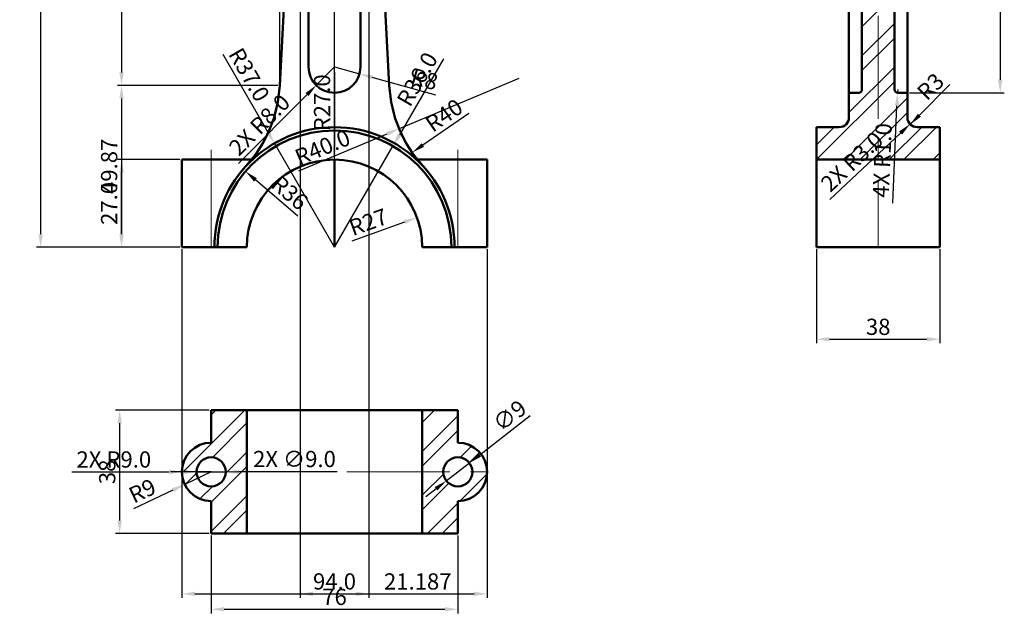
# Model space of a CAD drawing. Units: millimetres. Extents: x 3127 to 3430, y 1464 to 1830.
# Tile 1 of 2: x 3127 to 3430, y 1464 to 1647. Entities that reach past the tile are written whole.
import ezdxf

# ---------------------------------------------------------------- set-up
doc = ezdxf.new("R2010")
doc.units = ezdxf.units.MM
doc.linetypes.add('CENTER', pattern=[50.8, 31.75, -6.35, 6.35, -6.35])
for name, color, linetype, lineweight in [('M-CNTR', 1, 'CENTER', 18), ('M-DIMS', 2, 'Continuous', 25), ('M-HATC', 8, 'Continuous', 18), ('M-OUTL', 7, 'Continuous', 50)]:
    doc.layers.add(name, color=color, linetype=linetype, lineweight=lineweight)
doc.styles.get("Standard").update_dxf_attribs({"font": 'arial.ttf'})
doc.dimstyles.new('ISO-25', dxfattribs={"dimtxt": 5, "dimasz": 4, "dimexe": 1.25, "dimexo": 0.625, "dimtad": 1, "dimdsep": 46, "dimtxsty": 'Standard', "dimcen": 2.5, "dimadec": 0, "dimazin": 0, "dimtfac": 1, "dimtmove": 0, "dimatfit": 3, "dimfxl": 1, "dimarcsym": 0})

# ---------------------------------------------------------------- blocks, each defined once
blk = doc.blocks.new('*D1')
at = {"layer": 'Defpoints', "color": 0, "transparency": 16777216}
for p in [(3401.51, 1614.37), (3403.63, 1616.5)]:
    blk.add_point(p, dxfattribs=at)
at = {"layer": 'M-DIMS', "color": 0, "lineweight": -2, "transparency": 16777216}
blk.add_line((3413.75, 1626.62), (3404.34, 1617.2), dxfattribs=at)
at = {"layer": 'M-DIMS', "color": 0, "transparency": 16777216}
blk.add_solid([(3403.87, 1617.67), (3404.81, 1616.73), (3401.51, 1614.37)], dxfattribs=at)
at = {"layer": 'M-DIMS', "color": 0, "transparency": 16777216, "insert": (3408.21, 1625.57), "char_height": 5, "attachment_point": 5, "rotation": 45}
blk.add_mtext('R3', dxfattribs=at)
blk = doc.blocks.new('*D2')
at = {"layer": 'Defpoints', "color": 0, "transparency": 16777216}
for p in [(3372.63, 1576.5), (3410.63, 1576.5), (3410.63, 1548.12)]:
    blk.add_point(p, dxfattribs=at)
at = {"layer": 'M-DIMS', "color": 0, "lineweight": -2, "transparency": 16777216}
for p, q in [((3372.63, 1575.87), (3372.63, 1546.87)), ((3410.63, 1575.87), (3410.63, 1546.87)), ((3376.63, 1548.12), (3406.63, 1548.12))]:
    blk.add_line(p, q, dxfattribs=at)
at = {"layer": 'M-DIMS', "color": 0, "transparency": 16777216}
for points in [[(3376.63, 1548.78), (3376.63, 1547.45), (3372.63, 1548.12)], [(3406.63, 1548.78), (3406.63, 1547.45), (3410.63, 1548.12)]]:
    blk.add_solid(points, dxfattribs=at)
at = {"layer": 'M-DIMS', "color": 0, "transparency": 16777216, "insert": (3391.63, 1551.3), "char_height": 5, "attachment_point": 5}
blk.add_mtext('38', dxfattribs=at)
blk = doc.blocks.new('*D4')
at = {"layer": 'Defpoints', "color": 0, "transparency": 16777216}
for p in [(3186.15, 1488.22), (3262.15, 1488.22), (3262.15, 1464.86)]:
    blk.add_point(p, dxfattribs=at)
at = {"layer": 'M-DIMS', "color": 0, "lineweight": -2, "transparency": 16777216}
for p, q in [((3186.15, 1487.6), (3186.15, 1463.61)), ((3262.15, 1487.6), (3262.15, 1463.61)), ((3190.15, 1464.86), (3258.15, 1464.86))]:
    blk.add_line(p, q, dxfattribs=at)
at = {"layer": 'M-DIMS', "color": 0, "transparency": 16777216}
for points in [[(3190.15, 1465.53), (3190.15, 1464.2), (3186.15, 1464.86)], [(3258.15, 1465.53), (3258.15, 1464.2), (3262.15, 1464.86)]]:
    blk.add_solid(points, dxfattribs=at)
at = {"layer": 'M-DIMS', "color": 0, "transparency": 16777216, "insert": (3224.15, 1468.04), "char_height": 5, "attachment_point": 5}
blk.add_mtext('76', dxfattribs=at)
blk = doc.blocks.new('*D5')
at = {"layer": 'Defpoints', "color": 0, "transparency": 16777216}
for p in [(3186.15, 1526.22), (3157.96, 1488.22), (3186.15, 1488.22)]:
    blk.add_point(p, dxfattribs=at)
at = {"layer": 'M-DIMS', "color": 0, "lineweight": -2, "transparency": 16777216}
for p, q in [((3185.52, 1526.22), (3156.71, 1526.22)), ((3157.96, 1522.22), (3157.96, 1492.22)), ((3185.52, 1488.22), (3156.71, 1488.22))]:
    blk.add_line(p, q, dxfattribs=at)
at = {"layer": 'M-DIMS', "color": 0, "transparency": 16777216}
for points in [[(3157.29, 1522.22), (3158.63, 1522.22), (3157.96, 1526.22)], [(3157.29, 1492.22), (3158.63, 1492.22), (3157.96, 1488.22)]]:
    blk.add_solid(points, dxfattribs=at)
at = {"layer": 'M-DIMS', "color": 0, "transparency": 16777216, "insert": (3154.78, 1507.22), "char_height": 5, "attachment_point": 5, "rotation": 90}
blk.add_mtext('38', dxfattribs=at)
blk = doc.blocks.new('*D6')
at = {"layer": 'Defpoints', "color": 0, "transparency": 16777216}
for p in [(3186.15, 1507.22), (3178.02, 1503.36)]:
    blk.add_point(p, dxfattribs=at)
at = {"layer": 'M-DIMS', "color": 0, "lineweight": -2, "transparency": 16777216}
for p, q in [((3186.15, 1507.22), (3178.02, 1503.36)), ((3162.37, 1495.92), (3174.41, 1501.64))]:
    blk.add_line(p, q, dxfattribs=at)
at = {"layer": 'M-DIMS', "color": 0, "transparency": 16777216}
blk.add_solid([(3174.12, 1502.24), (3174.69, 1501.04), (3178.02, 1503.36)], dxfattribs=at)
at = {"layer": 'M-DIMS', "color": 0, "transparency": 16777216, "insert": (3165.22, 1500.79), "char_height": 5, "attachment_point": 5, "rotation": 25.423}
blk.add_mtext('R9', dxfattribs=at)
blk = doc.blocks.new('*D7')
at = {"layer": 'Defpoints', "color": 0, "transparency": 16777216}
for p in [(3265.71, 1509.98), (3258.59, 1504.47)]:
    blk.add_point(p, dxfattribs=at)
at = {"layer": 'M-DIMS', "color": 0, "lineweight": -2, "transparency": 16777216}
for p, q in [((3284.47, 1524.49), (3268.87, 1512.42)), ((3258.59, 1504.47), (3265.71, 1509.98)), ((3255.43, 1502.02), (3252.26, 1499.57))]:
    blk.add_line(p, q, dxfattribs=at)
at = {"layer": 'M-DIMS', "color": 0, "transparency": 16777216}
for points in [[(3268.46, 1512.95), (3269.28, 1511.9), (3265.71, 1509.98)], [(3255.02, 1502.55), (3255.83, 1501.49), (3258.59, 1504.47)]]:
    blk.add_solid(points, dxfattribs=at)
at = {"layer": 'M-DIMS', "color": 0, "transparency": 16777216, "insert": (3278.5, 1524.06), "char_height": 5, "attachment_point": 5, "rotation": 37.7248}
blk.add_mtext('∅9', dxfattribs=at)
blk = doc.blocks.new('*D8')
at = {"layer": 'Defpoints', "color": 0, "transparency": 16777216}
for p in [(3249.56, 1585.63), (3224.15, 1576.5)]:
    blk.add_point(p, dxfattribs=at)
at = {"layer": 'M-DIMS', "color": 0, "lineweight": -2, "transparency": 16777216}
blk.add_line((3229.61, 1578.46), (3245.79, 1584.28), dxfattribs=at)
at = {"layer": 'M-DIMS', "color": 0, "transparency": 16777216}
blk.add_solid([(3245.57, 1584.9), (3246.02, 1583.65), (3249.56, 1585.63)], dxfattribs=at)
at = {"layer": 'M-DIMS', "color": 0, "transparency": 16777216, "insert": (3234.76, 1583.64), "char_height": 5, "attachment_point": 5, "rotation": 19.7728}
blk.add_mtext('R27', dxfattribs=at)
blk = doc.blocks.new('*D9')
at = {"layer": 'Defpoints', "color": 0, "transparency": 16777216}
for p in [(3196.75, 1599.85), (3224.15, 1576.5)]:
    blk.add_point(p, dxfattribs=at)
at = {"layer": 'M-DIMS', "color": 0, "lineweight": -2, "transparency": 16777216}
blk.add_line((3212.88, 1586.1), (3199.79, 1597.25), dxfattribs=at)
at = {"layer": 'M-DIMS', "color": 0, "transparency": 16777216}
blk.add_solid([(3200.23, 1597.76), (3199.36, 1596.74), (3196.75, 1599.85)], dxfattribs=at)
at = {"layer": 'M-DIMS', "color": 0, "transparency": 16777216, "insert": (3209.92, 1592.8), "char_height": 5, "attachment_point": 5, "rotation": 319.5625}
blk.add_mtext('R36', dxfattribs=at)
blk = doc.blocks.new('*D10')
at = {"layer": 'Defpoints', "color": 0, "transparency": 16777216}
for p in [(3224.15, 1632.1), (3231.85, 1629.94)]:
    blk.add_point(p, dxfattribs=at)
at = {"layer": 'M-DIMS', "color": 0, "lineweight": -2, "transparency": 16777216}
for p, q in [((3224.15, 1632.1), (3231.85, 1629.94)), ((3255.34, 1623.37), (3235.71, 1628.86))]:
    blk.add_line(p, q, dxfattribs=at)
at = {"layer": 'M-DIMS', "color": 0, "transparency": 16777216}
blk.add_solid([(3235.88, 1629.51), (3235.53, 1628.22), (3231.85, 1629.94)], dxfattribs=at)
at = {"layer": 'M-DIMS', "color": 0, "transparency": 16777216, "insert": (3251.71, 1627.69), "char_height": 5, "attachment_point": 5, "rotation": 344.3775}
blk.add_mtext('R8', dxfattribs=at)
blk = doc.blocks.new('*D11')
at = {"layer": 'Defpoints', "color": 0, "transparency": 16777216}
for p in [(3280.97, 1628.46), (3248.08, 1605.7)]:
    blk.add_point(p, dxfattribs=at)
at = {"layer": 'M-DIMS', "color": 0, "lineweight": -2, "transparency": 16777216}
blk.add_line((3265.49, 1617.75), (3251.36, 1607.98), dxfattribs=at)
at = {"layer": 'M-DIMS', "color": 0, "transparency": 16777216}
blk.add_solid([(3250.99, 1608.53), (3251.74, 1607.43), (3248.08, 1605.7)], dxfattribs=at)
at = {"layer": 'M-DIMS', "color": 0, "transparency": 16777216, "insert": (3258.26, 1616.62), "char_height": 5, "attachment_point": 5, "rotation": 34.6821}
blk.add_mtext('R40', dxfattribs=at)
blk = doc.blocks.new('*D12')
at = {"layer": 'Defpoints', "color": 0, "transparency": 16777216}
for p in [(3213.56, 1746.21), (3234.74, 1746.21), (3219.51, 1682.41), (3207.27, 1626.37), (3241.02, 1626.37)]:
    blk.add_point(p, dxfattribs=at)
at = {"layer": 'M-DIMS', "color": 0, "lineweight": -2, "transparency": 16777216}
blk.add_arc((3224.15, 1948.35), 265.98, 267.8617, 272.1383, dxfattribs=at)
at = {"layer": 'M-DIMS', "color": 0, "transparency": 16777216}
for points in [[(3214.19, 1681.89), (3214.25, 1683.22), (3210.23, 1682.73)], [(3234.04, 1683.22), (3234.1, 1681.89), (3238.07, 1682.73)]]:
    blk.add_solid(points, dxfattribs=at)
at = {"layer": 'M-DIMS', "color": 0, "transparency": 16777216, "insert": (3224.15, 1685.55), "char_height": 5, "attachment_point": 5}
blk.add_mtext('6°', dxfattribs=at)
blk = doc.blocks.new('*D16')
at = {"layer": 'Defpoints', "color": 0, "transparency": 16777216}
for p in [(3224.15, 1777.7), (3133.63, 1576.5), (3177.15, 1576.5)]:
    blk.add_point(p, dxfattribs=at)
at = {"layer": 'M-DIMS', "color": 0, "lineweight": -2, "transparency": 16777216}
for p, q in [((3223.52, 1777.7), (3132.38, 1777.7)), ((3133.63, 1773.7), (3133.63, 1580.5)), ((3176.52, 1576.5), (3132.38, 1576.5))]:
    blk.add_line(p, q, dxfattribs=at)
at = {"layer": 'M-DIMS', "color": 0, "transparency": 16777216}
for points in [[(3132.96, 1773.7), (3134.3, 1773.7), (3133.63, 1777.7)], [(3132.96, 1580.5), (3134.3, 1580.5), (3133.63, 1576.5)]]:
    blk.add_solid(points, dxfattribs=at)
at = {"layer": 'M-DIMS', "color": 0, "transparency": 16777216, "insert": (3130.45, 1677.1), "char_height": 5, "attachment_point": 5, "rotation": 90}
blk.add_mtext('201.2', dxfattribs=at)
blk = doc.blocks.new('*D20')
at = {"layer": 'Defpoints', "color": 0, "transparency": 16777216}
for p in [(3177.15, 1576.5), (3271.15, 1576.5), (3271.15, 1469.62)]:
    blk.add_point(p, dxfattribs=at)
at = {"layer": 'M-DIMS', "color": 0, "lineweight": -2, "transparency": 16777216}
for p, q in [((3177.15, 1575.87), (3177.15, 1468.37)), ((3271.15, 1575.87), (3271.15, 1468.37)), ((3181.15, 1469.62), (3267.15, 1469.62))]:
    blk.add_line(p, q, dxfattribs=at)
at = {"layer": 'M-DIMS', "color": 0, "transparency": 16777216}
for points in [[(3181.15, 1470.29), (3181.15, 1468.96), (3177.15, 1469.62)], [(3267.15, 1470.29), (3267.15, 1468.96), (3271.15, 1469.62)]]:
    blk.add_solid(points, dxfattribs=at)
at = {"layer": 'M-DIMS', "color": 0, "transparency": 16777216, "insert": (3224.15, 1472.8), "char_height": 5, "attachment_point": 5}
blk.add_mtext('94.0', dxfattribs=at)
blk = doc.blocks.new('*D21')
at = {"layer": 'Defpoints', "color": 0, "transparency": 16777216}
for p in [(3158.55, 1603.5), (3177.15, 1603.5), (3177.15, 1576.5)]:
    blk.add_point(p, dxfattribs=at)
at = {"layer": 'M-DIMS', "color": 0, "lineweight": -2, "transparency": 16777216}
for p, q in [((3176.52, 1603.5), (3157.3, 1603.5)), ((3158.55, 1580.5), (3158.55, 1599.5)), ((3176.52, 1576.5), (3157.3, 1576.5))]:
    blk.add_line(p, q, dxfattribs=at)
at = {"layer": 'M-DIMS', "color": 0, "transparency": 16777216}
for points in [[(3157.88, 1599.5), (3159.22, 1599.5), (3158.55, 1603.5)], [(3157.88, 1580.5), (3159.22, 1580.5), (3158.55, 1576.5)]]:
    blk.add_solid(points, dxfattribs=at)
at = {"layer": 'M-DIMS', "color": 0, "transparency": 16777216, "insert": (3155.37, 1590), "char_height": 5, "attachment_point": 5, "rotation": 90}
blk.add_mtext('27.0', dxfattribs=at)
blk = doc.blocks.new('*D23')
at = {"layer": 'Defpoints', "color": 0, "transparency": 16777216}
for p in [(3400.63, 1730.1), (3400.63, 1624.1), (3429.23, 1624.1)]:
    blk.add_point(p, dxfattribs=at)
at = {"layer": 'M-DIMS', "color": 0, "lineweight": -2, "transparency": 16777216}
for p, q in [((3401.25, 1730.1), (3430.48, 1730.1)), ((3429.23, 1726.1), (3429.23, 1628.1)), ((3401.25, 1624.1), (3430.48, 1624.1))]:
    blk.add_line(p, q, dxfattribs=at)
at = {"layer": 'M-DIMS', "color": 0, "transparency": 16777216}
for points in [[(3428.56, 1726.1), (3429.9, 1726.1), (3429.23, 1730.1)], [(3428.56, 1628.1), (3429.9, 1628.1), (3429.23, 1624.1)]]:
    blk.add_solid(points, dxfattribs=at)
at = {"layer": 'M-DIMS', "color": 0, "transparency": 16777216, "insert": (3426.05, 1677.1), "char_height": 5, "attachment_point": 5, "rotation": 90}
blk.add_mtext('106.0', dxfattribs=at)
blk = doc.blocks.new('*D24')
at = {"layer": 'Defpoints', "color": 0, "transparency": 16777216}
for p in [(3213.56, 1746.21), (3234.74, 1746.21), (3234.74, 1469.62)]:
    blk.add_point(p, dxfattribs=at)
at = {"layer": 'M-DIMS', "color": 0, "lineweight": -2, "transparency": 16777216}
for p, q in [((3213.56, 1745.59), (3213.56, 1468.37)), ((3234.74, 1745.59), (3234.74, 1468.37)), ((3217.56, 1469.62), (3230.74, 1469.62)), ((3234.74, 1469.62), (3260.83, 1469.62))]:
    blk.add_line(p, q, dxfattribs=at)
at = {"layer": 'M-DIMS', "color": 0, "transparency": 16777216}
for points in [[(3217.56, 1470.29), (3217.56, 1468.96), (3213.56, 1469.62)], [(3230.74, 1470.29), (3230.74, 1468.96), (3234.74, 1469.62)]]:
    blk.add_solid(points, dxfattribs=at)
at = {"layer": 'M-DIMS', "color": 0, "transparency": 16777216, "insert": (3249.79, 1472.8), "char_height": 5, "attachment_point": 5}
blk.add_mtext('21.187', dxfattribs=at)
blk = doc.blocks.new('*D25')
at = {"layer": 'Defpoints', "color": 0, "transparency": 16777216}
for p in [(3224.15, 1818.8), (3207.27, 1626.37), (3224.15, 1603.5)]:
    blk.add_point(p, dxfattribs=at)
at = {"layer": 'M-DIMS', "color": 0, "lineweight": -2, "transparency": 16777216}
for p, q in [((3207.27, 1626.99), (3207.27, 1820.05)), ((3224.15, 1604.12), (3224.15, 1820.05)), ((3211.27, 1818.8), (3220.15, 1818.8)), ((3224.15, 1818.8), (3249.66, 1818.8))]:
    blk.add_line(p, q, dxfattribs=at)
at = {"layer": 'M-DIMS', "color": 0, "transparency": 16777216}
for points in [[(3211.27, 1819.46), (3211.27, 1818.13), (3207.27, 1818.8)], [(3220.15, 1819.46), (3220.15, 1818.13), (3224.15, 1818.8)]]:
    blk.add_solid(points, dxfattribs=at)
at = {"layer": 'M-DIMS', "color": 0, "transparency": 16777216, "insert": (3238.91, 1821.97), "char_height": 5, "attachment_point": 5}
blk.add_mtext('16.874', dxfattribs=at)
blk = doc.blocks.new('*D26')
at = {"layer": 'Defpoints', "color": 0, "transparency": 16777216}
for p in [(3213.56, 1746.21), (3158.55, 1626.37), (3207.27, 1626.37)]:
    blk.add_point(p, dxfattribs=at)
at = {"layer": 'M-DIMS', "color": 0, "lineweight": -2, "transparency": 16777216}
for p, q in [((3212.93, 1746.21), (3157.3, 1746.21)), ((3158.55, 1742.21), (3158.55, 1630.37)), ((3206.65, 1626.37), (3157.3, 1626.37))]:
    blk.add_line(p, q, dxfattribs=at)
at = {"layer": 'M-DIMS', "color": 0, "transparency": 16777216}
for points in [[(3157.88, 1742.21), (3159.22, 1742.21), (3158.55, 1746.21)], [(3157.88, 1630.37), (3159.22, 1630.37), (3158.55, 1626.37)]]:
    blk.add_solid(points, dxfattribs=at)
at = {"layer": 'M-DIMS', "color": 0, "transparency": 16777216, "insert": (3155.37, 1686.29), "char_height": 5, "attachment_point": 5, "rotation": 90}
blk.add_mtext('119.85', dxfattribs=at)
blk = doc.blocks.new('*D27')
at = {"layer": 'Defpoints', "color": 0, "transparency": 16777216}
for p in [(3207.27, 1626.37), (3158.55, 1576.5), (3177.15, 1576.5)]:
    blk.add_point(p, dxfattribs=at)
at = {"layer": 'M-DIMS', "color": 0, "lineweight": -2, "transparency": 16777216}
for p, q in [((3206.65, 1626.37), (3157.3, 1626.37)), ((3158.55, 1622.37), (3158.55, 1580.5)), ((3176.52, 1576.5), (3157.3, 1576.5))]:
    blk.add_line(p, q, dxfattribs=at)
at = {"layer": 'M-DIMS', "color": 0, "transparency": 16777216}
for points in [[(3157.88, 1622.37), (3159.22, 1622.37), (3158.55, 1626.37)], [(3157.88, 1580.5), (3159.22, 1580.5), (3158.55, 1576.5)]]:
    blk.add_solid(points, dxfattribs=at)
at = {"layer": 'M-DIMS', "color": 0, "transparency": 16777216, "insert": (3155.37, 1601.43), "char_height": 5, "attachment_point": 5, "rotation": 90}
blk.add_mtext('49.87', dxfattribs=at)
blk = doc.blocks.new('*D31')
at = {"layer": 'Defpoints', "color": 0, "transparency": 16777216}
for p in [(3224.15, 1632.1), (3218.52, 1626.42)]:
    blk.add_point(p, dxfattribs=at)
at = {"layer": 'M-DIMS', "color": 0, "lineweight": -2, "transparency": 16777216}
for p, q in [((3224.15, 1632.1), (3218.52, 1626.42)), ((3194.61, 1602.31), (3215.7, 1623.58))]:
    blk.add_line(p, q, dxfattribs=at)
at = {"layer": 'M-DIMS', "color": 0, "transparency": 16777216}
blk.add_solid([(3215.23, 1624.04), (3216.17, 1623.11), (3218.52, 1626.42)], dxfattribs=at)
at = {"layer": 'M-DIMS', "color": 0, "transparency": 16777216, "insert": (3201.49, 1613.76), "char_height": 5, "attachment_point": 5, "rotation": 45.2377}
blk.add_mtext('2X R8.0', dxfattribs=at)
blk = doc.blocks.new('*D32')
at = {"layer": 'Defpoints', "color": 0, "transparency": 16777216}
for p in [(3280.97, 1628.46), (3244.07, 1613.01)]:
    blk.add_point(p, dxfattribs=at)
at = {"layer": 'M-DIMS', "color": 0, "lineweight": -2, "transparency": 16777216}
for p, q in [((3280.97, 1628.46), (3244.07, 1613.01)), ((3213.17, 1600.07), (3240.38, 1611.47))]:
    blk.add_line(p, q, dxfattribs=at)
at = {"layer": 'M-DIMS', "color": 0, "transparency": 16777216}
blk.add_solid([(3240.13, 1612.08), (3240.64, 1610.85), (3244.07, 1613.01)], dxfattribs=at)
at = {"layer": 'M-DIMS', "color": 0, "transparency": 16777216, "insert": (3220.71, 1606.67), "char_height": 5, "attachment_point": 5, "rotation": 22.7235}
blk.add_mtext('R40.0', dxfattribs=at)
blk = doc.blocks.new('*D33')
at = {"layer": 'Defpoints', "color": 0, "transparency": 16777216}
for p in [(3205.65, 1608.54), (3224.15, 1576.5)]:
    blk.add_point(p, dxfattribs=at)
at = {"layer": 'M-DIMS', "color": 0, "lineweight": -2, "transparency": 16777216}
for p, q in [((3189.8, 1636), (3203.65, 1612)), ((3224.15, 1576.5), (3205.65, 1608.54))]:
    blk.add_line(p, q, dxfattribs=at)
at = {"layer": 'M-DIMS', "color": 0, "transparency": 16777216}
blk.add_solid([(3204.23, 1612.34), (3203.07, 1611.67), (3205.65, 1608.54)], dxfattribs=at)
at = {"layer": 'M-DIMS', "color": 0, "transparency": 16777216, "insert": (3197.3, 1629.36), "char_height": 5, "attachment_point": 5, "rotation": 299.9971}
blk.add_mtext('R37.0', dxfattribs=at)
blk = doc.blocks.new('*D34')
at = {"layer": 'Defpoints', "color": 0, "transparency": 16777216}
for p in [(3242.15, 1607.67), (3224.15, 1576.5)]:
    blk.add_point(p, dxfattribs=at)
at = {"layer": 'M-DIMS', "color": 0, "lineweight": -2, "transparency": 16777216}
for p, q in [((3257.7, 1634.61), (3244.15, 1611.14)), ((3224.15, 1576.5), (3242.15, 1607.67))]:
    blk.add_line(p, q, dxfattribs=at)
at = {"layer": 'M-DIMS', "color": 0, "transparency": 16777216}
blk.add_solid([(3243.57, 1611.47), (3244.72, 1610.8), (3242.15, 1607.67)], dxfattribs=at)
at = {"layer": 'M-DIMS', "color": 0, "transparency": 16777216, "insert": (3250.19, 1627.97), "char_height": 5, "attachment_point": 5, "rotation": 60.004}
blk.add_mtext('R36.0', dxfattribs=at)
blk = doc.blocks.new('*D35')
at = {"layer": 'Defpoints', "color": 0, "transparency": 16777216}
for p in [(3224.15, 1603.5), (3224.15, 1576.5)]:
    blk.add_point(p, dxfattribs=at)
at = {"layer": 'M-DIMS', "color": 0, "lineweight": -2, "transparency": 16777216}
for p, q in [((3224.15, 1630.5), (3224.15, 1607.5)), ((3224.15, 1576.5), (3224.15, 1603.5))]:
    blk.add_line(p, q, dxfattribs=at)
at = {"layer": 'M-DIMS', "color": 0, "transparency": 16777216}
blk.add_solid([(3223.48, 1607.5), (3224.82, 1607.5), (3224.15, 1603.5)], dxfattribs=at)
at = {"layer": 'M-DIMS', "color": 0, "transparency": 16777216, "insert": (3220.97, 1621), "char_height": 5, "attachment_point": 5, "rotation": 89.9992}
blk.add_mtext('R27.0', dxfattribs=at)
blk = doc.blocks.new('*D36')
at = {"layer": 'Defpoints', "color": 0, "transparency": 16777216}
for p in [(3177.15, 1507.22), (3186.15, 1507.22)]:
    blk.add_point(p, dxfattribs=at)
at = {"layer": 'M-DIMS', "color": 0, "lineweight": -2, "transparency": 16777216}
for p, q in [((3143.2, 1507.22), (3173.15, 1507.22)), ((3186.15, 1507.22), (3177.15, 1507.22))]:
    blk.add_line(p, q, dxfattribs=at)
at = {"layer": 'M-DIMS', "color": 0, "transparency": 16777216}
blk.add_solid([(3173.15, 1507.89), (3173.15, 1506.56), (3177.15, 1507.22)], dxfattribs=at)
at = {"layer": 'M-DIMS', "color": 0, "transparency": 16777216, "insert": (3156.17, 1510.4), "char_height": 5, "attachment_point": 5, "rotation": 359.9991}
blk.add_mtext('2X R9.0', dxfattribs=at)
blk = doc.blocks.new('*D37')
at = {"layer": 'Defpoints', "color": 0, "transparency": 16777216}
for p in [(3181.65, 1507.22), (3190.65, 1507.22)]:
    blk.add_point(p, dxfattribs=at)
at = {"layer": 'M-DIMS', "color": 0, "lineweight": -2, "transparency": 16777216}
for p, q in [((3177.65, 1507.22), (3173.65, 1507.22)), ((3181.65, 1507.22), (3190.65, 1507.22)), ((3224.99, 1507.22), (3194.65, 1507.22))]:
    blk.add_line(p, q, dxfattribs=at)
at = {"layer": 'M-DIMS', "color": 0, "transparency": 16777216}
for points in [[(3177.65, 1507.89), (3177.65, 1506.55), (3181.65, 1507.22)], [(3194.65, 1507.89), (3194.65, 1506.56), (3190.65, 1507.22)]]:
    blk.add_solid(points, dxfattribs=at)
at = {"layer": 'M-DIMS', "color": 0, "transparency": 16777216, "insert": (3211.82, 1510.54), "char_height": 5, "attachment_point": 5, "rotation": 0.0018}
blk.add_mtext('2X ∅9.0', dxfattribs=at)
blk = doc.blocks.new('*D38')
at = {"layer": 'Defpoints', "color": 0, "transparency": 16777216}
for p in [(3401.44, 1614.44), (3403.63, 1616.5)]:
    blk.add_point(p, dxfattribs=at)
at = {"layer": 'M-DIMS', "color": 0, "lineweight": -2, "transparency": 16777216}
for p, q in [((3403.63, 1616.5), (3401.44, 1614.44)), ((3376.71, 1591.19), (3398.53, 1611.7))]:
    blk.add_line(p, q, dxfattribs=at)
at = {"layer": 'M-DIMS', "color": 0, "transparency": 16777216}
blk.add_solid([(3398.07, 1612.19), (3398.99, 1611.22), (3401.44, 1614.44)], dxfattribs=at)
at = {"layer": 'M-DIMS', "color": 0, "transparency": 16777216, "insert": (3383.98, 1602.39), "char_height": 5, "attachment_point": 5, "rotation": 43.2283}
blk.add_mtext('2X R3.0', dxfattribs=at)
blk = doc.blocks.new('*D39')
at = {"layer": 'Defpoints', "color": 0, "transparency": 16777216}
for p in [(3397.59, 1624.1), (3397.63, 1625.1)]:
    blk.add_point(p, dxfattribs=at)
at = {"layer": 'M-DIMS', "color": 0, "lineweight": -2, "transparency": 16777216}
for p, q in [((3397.63, 1625.1), (3397.59, 1624.1)), ((3396.14, 1590.06), (3397.42, 1620.1))]:
    blk.add_line(p, q, dxfattribs=at)
at = {"layer": 'M-DIMS', "color": 0, "transparency": 16777216}
blk.add_solid([(3396.75, 1620.13), (3398.08, 1620.07), (3397.59, 1624.1)], dxfattribs=at)
at = {"layer": 'M-DIMS', "color": 0, "transparency": 16777216, "insert": (3393.52, 1603.22), "char_height": 5, "attachment_point": 5, "rotation": 87.5733}
blk.add_mtext('4X R1.0', dxfattribs=at)

msp = doc.modelspace()

# ---------------------------------------------------------------- hatches: boundary and pattern name
at = {"layer": 'M-HATC'}
h = msp.add_hatch(dxfattribs=at)
h.set_pattern_fill('ANSI32', color=256)
h.paths.add_polyline_path([(3391.6295, 1800.1957), (3372.6295, 1800.1957), (3372.6295, 1794.5957), (3391.6295, 1794.5957)])
h.paths.add_polyline_path([(3410.6295, 1800.1957), (3391.6295, 1800.1957), (3391.6295, 1794.5957), (3410.6295, 1794.5957)])
h.paths.add_polyline_path([(3400.6295, 1755.1957), (3410.6295, 1755.1957), (3410.6295, 1760.7957), (3391.6295, 1760.7957), (3391.6295, 1603.4957), (3410.6295, 1603.4957), (3410.6295, 1613.4957), (3403.6295, 1613.4957, -0.41421356), (3400.6295, 1616.4957), (3400.6295, 1624.0957), (3397.6295, 1624.0957, -0.41421356), (3396.6295, 1625.0957), (3396.6295, 1729.0957, -0.41421356), (3397.6295, 1730.0957), (3400.6295, 1730.0957)])
h.paths.add_polyline_path([(3391.6295, 1760.7957), (3372.6295, 1760.7957), (3372.6295, 1755.1957), (3382.6295, 1755.1957), (3382.6295, 1730.0957), (3385.6295, 1730.0957, -0.41421356), (3386.6295, 1729.0957), (3386.6295, 1625.0957, -0.41421356), (3385.6295, 1624.0957), (3382.6295, 1624.0957), (3382.6295, 1616.4957, -0.41421356), (3379.6295, 1613.4957), (3372.6295, 1613.4957), (3372.6295, 1603.4957), (3391.6295, 1603.4957)])
h.paths.add_polyline_path([(3262.1486, 1526.2219), (3251.1486, 1526.2219), (3251.1486, 1507.2219), (3257.6486, 1507.2219, -1), (3266.6486, 1507.2219), (3271.1486, 1507.2219, 0.41421356), (3262.1486, 1516.2219)])
h.paths.add_polyline_path([(3271.1486, 1507.2219), (3266.6486, 1507.2219, -1), (3257.6486, 1507.2219), (3251.1486, 1507.2219), (3251.1486, 1488.2219), (3262.1486, 1488.2219), (3262.1486, 1498.2219, 0.41421356)])
h.paths.add_polyline_path([(3197.1486, 1526.2219), (3186.1486, 1526.2219), (3186.1486, 1516.2219, 0.41421356), (3177.1486, 1507.2219), (3181.6486, 1507.2219, -1), (3190.6486, 1507.2219), (3197.1486, 1507.2219)])
h.paths.add_polyline_path([(3197.1486, 1507.2219), (3190.6486, 1507.2219, -1), (3181.6486, 1507.2219), (3177.1486, 1507.2219, 0.41421356), (3186.1486, 1498.2219), (3186.1486, 1488.2219), (3197.1486, 1488.2219)])

# ---------------------------------------------------------------- linework, layer by layer
at = {"layer": 'M-CNTR'}
for p, q in [((3391.6295, 1800.1957), (3391.6295, 1576.4957)), ((3224.1486, 1777.6957), (3224.1486, 1624.0957)), ((3224.1486, 1624.0957), (3224.1486, 1576.4957)), ((3186.1486, 1576.4957), (3186.1486, 1606.4957)), ((3262.1486, 1576.4957), (3262.1486, 1606.4957)), ((3177.1486, 1507.2219), (3271.1486, 1507.2219))]:
    msp.add_line(p, q, dxfattribs=at)
at = {"layer": 'M-OUTL'}
for p, q in [((3382.6295, 1755.1957), (3382.6295, 1616.4957)), ((3400.6295, 1755.1957), (3400.6295, 1616.4957)), ((3213.5551, 1746.2148), (3207.2742, 1626.369)), ((3234.7422, 1746.2148), (3241.023, 1626.369)), ((3386.6295, 1729.0957), (3386.6295, 1625.0957)), ((3396.6295, 1729.0957), (3396.6295, 1625.0957)), ((3216.1486, 1722.0957), (3216.1486, 1632.0957)), ((3232.1486, 1722.0957), (3232.1486, 1632.0957)), ((3382.6295, 1624.0957), (3385.6295, 1624.0957)), ((3397.6295, 1624.0957), (3400.6295, 1624.0957)), ((3372.6295, 1613.4957), (3372.6295, 1576.4957)), ((3372.6295, 1613.4957), (3379.6295, 1613.4957)), ((3403.6295, 1613.4957), (3410.6295, 1613.4957)), ((3410.6295, 1613.4957), (3410.6295, 1576.4957)), ((3177.1486, 1576.4957), (3177.1486, 1603.4957)), ((3177.1486, 1603.4957), (3198.5807, 1603.4957)), ((3224.1486, 1576.4957), (3224.1486, 1603.4957)), ((3249.7166, 1603.4957), (3271.1486, 1603.4957)), ((3249.7166, 1603.4957), (3271.1486, 1603.4957)), ((3271.1486, 1576.4957), (3271.1486, 1603.4957)), ((3372.6295, 1603.4957), (3410.6295, 1603.4957)), ((3177.1486, 1576.4957), (3197.1486, 1576.4957)), ((3187.1486, 1576.4957), (3197.1486, 1576.4957)), ((3251.1486, 1576.4957), (3261.1486, 1576.4957)), ((3251.1486, 1576.4957), (3271.1486, 1576.4957)), ((3251.1486, 1576.4957), (3271.1486, 1576.4957)), ((3372.6295, 1576.4957), (3410.6295, 1576.4957)), ((3186.1486, 1526.2219), (3262.1486, 1526.2219)), ((3186.1486, 1516.2219), (3186.1486, 1526.2219)), ((3197.1486, 1526.2219), (3197.1486, 1488.2219)), ((3251.1486, 1526.2219), (3251.1486, 1488.2219)), ((3262.1486, 1516.2219), (3262.1486, 1526.2219)), ((3186.1486, 1488.2219), (3186.1486, 1498.2219)), ((3262.1486, 1488.2219), (3262.1486, 1498.2219)), ((3186.1486, 1488.2219), (3262.1486, 1488.2219))]:
    msp.add_line(p, q, dxfattribs=at)
for centre in [(3186.1486, 1507.2219), (3262.1486, 1507.2219)]:
    msp.add_circle(centre, 4.5, dxfattribs=at)
for centre, radius, start, end in [((3224.1486, 1632.0957), 8, 180, 0), ((3167.3291, 1628.4624), 40, 317.554231, 357), ((3280.9682, 1628.4624), 40, 183, 222.445769), ((3385.6295, 1625.0957), 1, 270, 0), ((3397.6295, 1625.0957), 1, 180, 270), ((3379.6295, 1616.4957), 3, 270, 0), ((3403.6295, 1616.4957), 3, 180, 270), ((3224.1486, 1576.4957), 37, 0, 180), ((3224.1486, 1576.4957), 36, 0, 180), ((3224.1486, 1576.4957), 27, 0, 180), ((3186.1486, 1507.2219), 9, 90, 270), ((3262.1486, 1507.2219), 9, 270, 90)]:
    msp.add_arc(centre, radius, start, end, dxfattribs=at)

# ---------------------------------------------------------------- dimensions: what is measured, and where the dimension line sits
at = {"layer": 'M-DIMS'}
for base, p1, p2, override, picture, middle in [((3224.1486, 1818.7957), (3207.2742, 1626.369), (3224.1486, 1603.4957), {"dimdec": 3, "dimlfac": 1, "dimrnd": 0, "dimzin": 0, "dimdsep": 46, "dimlunit": 2}, '*D25', (3238.9067, 1821.9736)), ((3234.7422, 1469.6219), (3213.5551, 1746.2148), (3234.7422, 1746.2148), {"dimdec": 3, "dimlfac": 1, "dimrnd": 0, "dimzin": 0, "dimdsep": 46, "dimlunit": 2}, '*D24', (3249.7884, 1472.7997)), ((3271.1486, 1469.6219), (3177.1486, 1576.4957), (3271.1486, 1576.4957), {"dimdec": 1, "dimlfac": 1, "dimrnd": 0, "dimzin": 0, "dimdsep": 46, "dimlunit": 2}, '*D20', (3224.1486, 1472.7997)), ((3410.6295, 1548.117), (3372.6295, 1576.4957), (3410.6295, 1576.4957), {"dimclrd": 0, "dimclre": 0, "dimclrt": 0}, '*D2', (3391.6295, 1551.2966)), ((3262.1486, 1464.8644), (3186.1486, 1488.2219), (3262.1486, 1488.2219), {"dimclrd": 0, "dimclre": 0, "dimclrt": 0}, '*D4', (3224.1486, 1468.0423))]:
    dim = msp.add_linear_dim(base=base, p1=p1, p2=p2, dimstyle='ISO-25', override=override, dxfattribs=at)
    dim.commit()
    dim.dimension.update_dxf_attribs({"geometry": picture, "text_midpoint": middle})
for base, p1, p2, override, picture, middle in [((3133.6315, 1576.4957), (3224.1486, 1777.6957), (3177.1486, 1576.4957), {"dimclrd": 0, "dimclre": 0, "dimclrt": 0}, '*D16', (3130.4537, 1677.0957)), ((3158.5486, 1626.369), (3213.5551, 1746.2148), (3207.2742, 1626.369), {"dimdec": 2, "dimlfac": 1, "dimrnd": 0, "dimzin": 0, "dimdsep": 46, "dimlunit": 2}, '*D26', (3155.3708, 1686.2919)), ((3429.2295, 1624.0957), (3400.6295, 1730.0957), (3400.6295, 1624.0957), {"dimdec": 1, "dimlfac": 1, "dimrnd": 0, "dimzin": 0, "dimdsep": 46, "dimlunit": 2}, '*D23', (3426.0516, 1677.0957)), ((3158.5486, 1576.4957), (3207.2742, 1626.369), (3177.1486, 1576.4957), {"dimdec": 2, "dimlfac": 1, "dimrnd": 0, "dimzin": 0, "dimdsep": 46, "dimlunit": 2}, '*D27', (3155.3708, 1601.4323)), ((3158.5486, 1603.4957), (3177.1486, 1576.4957), (3177.1486, 1603.4957), {"dimdec": 1, "dimlfac": 1, "dimrnd": 0, "dimzin": 0, "dimdsep": 46, "dimlunit": 2}, '*D21', (3155.3708, 1589.9957)), ((3157.9612, 1488.2219), (3186.1486, 1526.2219), (3186.1486, 1488.2219), {"dimclrd": 0, "dimclre": 0, "dimclrt": 0}, '*D5', (3154.7816, 1507.2219))]:
    dim = msp.add_linear_dim(base=base, p1=p1, p2=p2, angle=90, dimstyle='ISO-25', override=override, dxfattribs=at)
    dim.commit()
    dim.dimension.update_dxf_attribs({"geometry": picture, "text_midpoint": middle})
dim = msp.add_angular_dim_2l(base=(3219.5066, 1682.4079), line1=((3234.7422, 1746.2148), (3241.023, 1626.369)), line2=((3213.5551, 1746.2148), (3207.2742, 1626.369)), dimstyle='ISO-25', override={"dimclrd": 0, "dimclre": 0, "dimclrt": 0}, dxfattribs=at)
dim.commit()
dim.dimension.update_dxf_attribs({"geometry": '*D12', "text_midpoint": (3224.1486, 1685.5453)})
for center, mpoint, override, picture, middle in [((3224.1486, 1576.4957), (3205.6502, 1608.5396), {"dimdec": 1, "dimlfac": 1, "dimrnd": 0, "dimzin": 0, "dimdsep": 46, "dimlunit": 2}, '*D33', (3194.5512, 1627.7659)), ((3224.1486, 1576.4957), (3242.1465, 1607.6739), {"dimdec": 1, "dimlfac": 1, "dimrnd": 0, "dimzin": 0, "dimdsep": 46, "dimlunit": 2}, '*D34', (3252.9452, 1626.3808)), ((3224.1486, 1632.0957), (3231.8531, 1629.9413), {"dimclrd": 0, "dimclre": 0, "dimclrt": 0}, '*D10', (3250.8507, 1624.629)), ((3403.6295, 1616.4957), (3401.5082, 1614.3744), {"dimclrd": 0, "dimclre": 0, "dimclrt": 0}, '*D1', (3410.4576, 1623.3238)), ((3280.9682, 1628.4624), (3244.073, 1613.011), {"dimdec": 1, "dimlfac": 1, "dimrnd": 0, "dimzin": 0, "dimdsep": 46, "dimlunit": 2}, '*D32', (3221.9359, 1603.7402)), ((3280.9682, 1628.4624), (3248.0753, 1605.7015), {"dimclrd": 0, "dimclre": 0, "dimclrt": 0}, '*D11', (3260.0732, 1614.0037)), ((3224.1486, 1576.4957), (3196.7485, 1599.846), {"dimclrd": 0, "dimclre": 0, "dimclrt": 0}, '*D9', (3207.8585, 1590.3781)), ((3224.1486, 1576.4957), (3249.5568, 1585.6296), {"dimclrd": 0, "dimclre": 0, "dimclrt": 0}, '*D8', (3235.8187, 1580.6909))]:
    dim = msp.add_radius_dim(center=center, mpoint=mpoint, dimstyle='ISO-25', override=override, dxfattribs=at)
    dim.commit()
    dim.dimension.update_dxf_attribs({"geometry": picture, "text_midpoint": middle, "dimtype": 164})
for center, mpoint, text, picture, middle in [((3224.1486, 1632.0957), (3218.5153, 1626.4154), '2X <>', '*D31', (3201.489, 1613.7603)), ((3397.6295, 1625.0957), (3397.5871, 1624.0966), '4X <>', '*D39', (3393.5216, 1603.2171)), ((3403.6295, 1616.4957), (3401.4436, 1614.441), '2X <>', '*D38', (3383.9829, 1602.3918)), ((3186.1486, 1507.2219), (3177.1486, 1507.222), '2X <>', '*D36', (3156.1738, 1510.4002))]:
    dim = msp.add_radius_dim(center=center, mpoint=mpoint, text=text, dimstyle='ISO-25', override={"dimdec": 1, "dimlfac": 1, "dimrnd": 0, "dimzin": 0, "dimdsep": 46, "dimlunit": 2}, dxfattribs=at)
    dim.commit()
    dim.dimension.update_dxf_attribs({"geometry": picture, "text_midpoint": middle})
for center, mpoint, override, picture, middle in [((3224.1486, 1576.4957), (3224.149, 1603.4957), {"dimdec": 1, "dimlfac": 1, "dimrnd": 0, "dimzin": 0, "dimdsep": 46, "dimlunit": 2}, '*D35', (3220.9714, 1620.9986)), ((3186.1486, 1507.2219), (3178.0202, 1503.3582), {"dimclrd": 0, "dimclre": 0, "dimclrt": 0}, '*D6', (3165.2205, 1500.7928))]:
    dim = msp.add_radius_dim(center=center, mpoint=mpoint, dimstyle='ISO-25', override=override, dxfattribs=at)
    dim.commit()
    dim.dimension.update_dxf_attribs({"geometry": picture, "text_midpoint": middle})
dim = msp.add_diameter_dim_2p(p1=(3258.5893, 1504.4684), p2=(3265.7079, 1509.9753), dimstyle='ISO-25', override={"dimclrd": 0, "dimclre": 0, "dimclrt": 0}, dxfattribs=at)
dim.commit()
dim.dimension.update_dxf_attribs({"geometry": '*D7', "text_midpoint": (3280.526, 1521.4383), "dimtype": 163})
dim = msp.add_diameter_dim_2p(p1=(3181.6486, 1507.2217), p2=(3190.6486, 1507.222), text='2X <>', dimstyle='ISO-25', override={"dimdec": 1, "dimlfac": 1, "dimrnd": 0, "dimzin": 0, "dimdsep": 46, "dimlunit": 2}, dxfattribs=at)
dim.commit()
dim.dimension.update_dxf_attribs({"geometry": '*D37', "text_midpoint": (3211.818, 1507.2227)})

doc.saveas('drawing.dxf')
